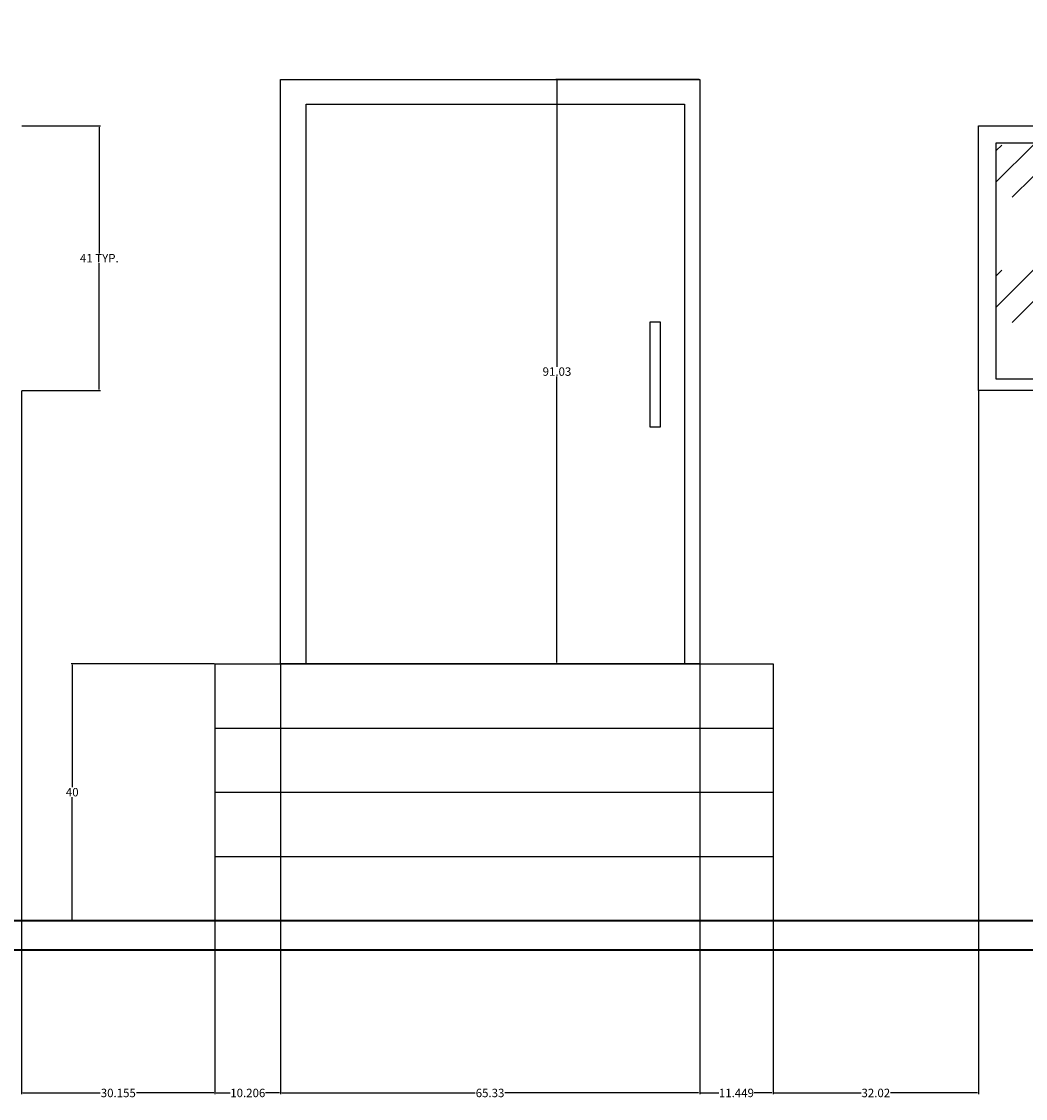
# Model space of a CAD drawing. Units: inches. Extents: x 30 to 515, y 94 to 489.
# Tile 4 of 7: x 202 to 358, y 94 to 262. Entities that reach past the tile are written whole.
import ezdxf

# ---------------------------------------------------------------- set-up
doc = ezdxf.new("R2010")
doc.units = ezdxf.units.IN
doc.header["$MEASUREMENT"] = 0
for name, color, linetype, lineweight in [('A-ANNO-DIMS', 2, 'Continuous', 18), ('A-DOOR', 4, 'Continuous', 25), ('A-FLOR-STRS', 3, 'Continuous', 25), ('A-GLAZ', 4, 'Continuous', 25), ('A-GLAZ-PATT', 8, 'Continuous', 13), ('A-WALL', 7, 'Continuous', 35)]:
    doc.layers.add(name, color=color, linetype=linetype, lineweight=lineweight)
doc.styles.get("Standard").update_dxf_attribs({"font": 'arial.ttf'})
doc.dimstyles.get("Standard").update_dxf_attribs({"dimtxt": 1.3125, "dimasz": 0.18, "dimexe": 0.18, "dimexo": 0.0625, "dimgap": 0.09, "dimtad": 0, "dimtih": 1, "dimtoh": 1, "dimdec": 4, "dimzin": 0, "dimdsep": 46, "dimlunit": 4, "dimtxsty": 'Standard', "dimcen": 0.09, "dimadec": 0, "dimazin": 0, "dimtfac": 1, "dimtdec": 4, "dimtofl": 0, "dimtmove": 0, "dimatfit": 3, "dimfxl": 1, "dimtolj": 1, "dimtzin": 0, "dimarcsym": 0})

# ---------------------------------------------------------------- blocks, each defined once
blk = doc.blocks.new('WIN-1100-DBL')
for points in [[(0, 41.22), (80.81, 41.22), (80.81, 0), (0, 0)], [(2.73, 38.58), (38.51, 38.58), (38.51, 1.75), (2.73, 1.75)], [(42.07, 38.58), (77.85, 38.58), (77.85, 1.75), (42.07, 1.75)], [(36.99, 20.89), (37.45, 20.89), (37.45, 13.69), (36.99, 13.69)], [(43.35, 20.89), (43.81, 20.89), (43.81, 13.69), (43.35, 13.69)]]:
    blk.add_lwpolyline(points, close=True)
blk = doc.blocks.new('*D3')
at = {"layer": 'A-ANNO-DIMS', "color": 0, "lineweight": -2, "transparency": 16777216}
for p, q in [((201.86, 245.32), (214.1, 245.32)), ((213.92, 245.14), (213.92, 225.45)), ((213.92, 204.27), (213.92, 223.96)), ((201.86, 204.09), (214.1, 204.09))]:
    blk.add_line(p, q, dxfattribs=at)
at = {"layer": 'A-ANNO-DIMS', "color": 0, "transparency": 16777216}
for points in [[(213.89, 245.14), (213.95, 245.14), (213.92, 245.32)], [(213.89, 204.27), (213.95, 204.27), (213.92, 204.09)]]:
    blk.add_solid(points, dxfattribs=at)
at = {"layer": 'Defpoints', "color": 0, "transparency": 16777216}
for p in [(201.8, 245.32), (213.92, 245.32), (201.8, 204.09)]:
    blk.add_point(p, dxfattribs=at)
at = {"layer": 'A-ANNO-DIMS', "color": 0, "transparency": 16777216, "insert": (213.92, 224.71), "char_height": 1.3125, "attachment_point": 5}
blk.add_mtext('\\A1;41 TYP.', dxfattribs=at)
blk = doc.blocks.new('*D8')
at = {"layer": 'A-ANNO-DIMS', "color": 0, "lineweight": -2, "transparency": 16777216}
for p, q in [((201.8, 204.03), (201.8, 94.5)), ((231.95, 121.47), (231.95, 94.5)), ((201.98, 94.68), (214.06, 94.68)), ((231.77, 94.68), (219.69, 94.68))]:
    blk.add_line(p, q, dxfattribs=at)
at = {"layer": 'A-ANNO-DIMS', "color": 0, "transparency": 16777216}
for points in [[(201.98, 94.71), (201.98, 94.65), (201.8, 94.68)], [(231.77, 94.71), (231.77, 94.65), (231.95, 94.68)]]:
    blk.add_solid(points, dxfattribs=at)
at = {"layer": 'Defpoints', "color": 0, "transparency": 16777216}
for p in [(201.8, 204.09), (231.95, 121.53), (231.95, 94.68)]:
    blk.add_point(p, dxfattribs=at)
at = {"layer": 'A-ANNO-DIMS', "color": 0, "transparency": 16777216, "insert": (216.88, 94.68), "char_height": 1.312, "attachment_point": 5}
blk.add_mtext('\\A1;30.155', dxfattribs=at)
blk = doc.blocks.new('*D9')
at = {"layer": 'A-ANNO-DIMS', "color": 0, "lineweight": -2, "transparency": 16777216}
for p, q in [((242.16, 161.47), (242.16, 94.5)), ((231.95, 121.47), (231.95, 94.5)), ((232.13, 94.68), (234.3, 94.68)), ((241.98, 94.68), (239.81, 94.68))]:
    blk.add_line(p, q, dxfattribs=at)
at = {"layer": 'A-ANNO-DIMS', "color": 0, "transparency": 16777216}
for points in [[(232.13, 94.71), (232.13, 94.65), (231.95, 94.68)], [(241.98, 94.71), (241.98, 94.65), (242.16, 94.68)]]:
    blk.add_solid(points, dxfattribs=at)
at = {"layer": 'Defpoints', "color": 0, "transparency": 16777216}
for p in [(242.16, 161.53), (231.95, 121.53), (242.16, 94.68)]:
    blk.add_point(p, dxfattribs=at)
at = {"layer": 'A-ANNO-DIMS', "color": 0, "transparency": 16777216, "insert": (237.06, 94.68), "char_height": 1.312, "attachment_point": 5}
blk.add_mtext('\\A1;10.206', dxfattribs=at)
blk = doc.blocks.new('*D10')
at = {"layer": 'A-ANNO-DIMS', "color": 0, "lineweight": -2, "transparency": 16777216}
for p, q in [((242.16, 161.47), (242.16, 94.5)), ((307.49, 161.47), (307.49, 94.5)), ((242.34, 94.68), (272.51, 94.68)), ((307.31, 94.68), (277.13, 94.68))]:
    blk.add_line(p, q, dxfattribs=at)
at = {"layer": 'A-ANNO-DIMS', "color": 0, "transparency": 16777216}
for points in [[(242.34, 94.71), (242.34, 94.65), (242.16, 94.68)], [(307.31, 94.71), (307.31, 94.65), (307.49, 94.68)]]:
    blk.add_solid(points, dxfattribs=at)
at = {"layer": 'Defpoints', "color": 0, "transparency": 16777216}
for p in [(242.16, 161.53), (307.49, 161.53), (307.49, 94.68)]:
    blk.add_point(p, dxfattribs=at)
at = {"layer": 'A-ANNO-DIMS', "color": 0, "transparency": 16777216, "insert": (274.82, 94.68), "char_height": 1.312, "attachment_point": 5}
blk.add_mtext('\\A1;65.33', dxfattribs=at)
blk = doc.blocks.new('*D11')
at = {"layer": 'A-ANNO-DIMS', "color": 0, "lineweight": -2, "transparency": 16777216}
for p, q in [((307.49, 161.47), (307.49, 94.5)), ((318.93, 121.47), (318.93, 94.5)), ((307.67, 94.68), (310.46, 94.68)), ((318.75, 94.68), (315.96, 94.68))]:
    blk.add_line(p, q, dxfattribs=at)
at = {"layer": 'A-ANNO-DIMS', "color": 0, "transparency": 16777216}
for points in [[(307.67, 94.71), (307.67, 94.65), (307.49, 94.68)], [(318.75, 94.71), (318.75, 94.65), (318.93, 94.68)]]:
    blk.add_solid(points, dxfattribs=at)
at = {"layer": 'Defpoints', "color": 0, "transparency": 16777216}
for p in [(307.49, 161.53), (318.93, 121.53), (318.93, 94.68)]:
    blk.add_point(p, dxfattribs=at)
at = {"layer": 'A-ANNO-DIMS', "color": 0, "transparency": 16777216, "insert": (313.21, 94.68), "char_height": 1.312, "attachment_point": 5}
blk.add_mtext('\\A1;11.449', dxfattribs=at)
blk = doc.blocks.new('*D12')
at = {"layer": 'A-ANNO-DIMS', "color": 0, "lineweight": -2, "transparency": 16777216}
for p, q in [((350.95, 204.03), (350.95, 94.5)), ((318.93, 121.47), (318.93, 94.5)), ((319.11, 94.68), (332.65, 94.68)), ((350.77, 94.68), (337.24, 94.68))]:
    blk.add_line(p, q, dxfattribs=at)
at = {"layer": 'A-ANNO-DIMS', "color": 0, "transparency": 16777216}
for points in [[(319.11, 94.71), (319.11, 94.65), (318.93, 94.68)], [(350.77, 94.71), (350.77, 94.65), (350.95, 94.68)]]:
    blk.add_solid(points, dxfattribs=at)
at = {"layer": 'Defpoints', "color": 0, "transparency": 16777216}
for p in [(350.95, 204.09), (318.93, 121.53), (350.95, 94.68)]:
    blk.add_point(p, dxfattribs=at)
at = {"layer": 'A-ANNO-DIMS', "color": 0, "transparency": 16777216, "insert": (334.94, 94.68), "char_height": 1.312, "attachment_point": 5}
blk.add_mtext('\\A1;32.02', dxfattribs=at)
blk = doc.blocks.new('*D28')
at = {"layer": 'A-ANNO-DIMS', "color": 0, "lineweight": -2, "transparency": 16777216}
for p, q in [((231.89, 161.53), (209.52, 161.53)), ((209.7, 161.35), (209.7, 142.29)), ((209.7, 121.71), (209.7, 140.77)), ((231.89, 121.53), (209.52, 121.53))]:
    blk.add_line(p, q, dxfattribs=at)
at = {"layer": 'A-ANNO-DIMS', "color": 0, "transparency": 16777216}
for points in [[(209.67, 161.35), (209.73, 161.35), (209.7, 161.53)], [(209.67, 121.71), (209.73, 121.71), (209.7, 121.53)]]:
    blk.add_solid(points, dxfattribs=at)
at = {"layer": 'Defpoints', "color": 0, "transparency": 16777216}
for p in [(209.7, 161.53), (231.95, 161.53), (231.95, 121.53)]:
    blk.add_point(p, dxfattribs=at)
at = {"layer": 'A-ANNO-DIMS', "color": 0, "transparency": 16777216, "insert": (209.7, 141.53), "char_height": 1.312, "attachment_point": 5}
blk.add_mtext('\\A1;40', dxfattribs=at)
blk = doc.blocks.new('*D29')
at = {"layer": 'A-ANNO-DIMS', "color": 0, "lineweight": -2, "transparency": 16777216}
for p, q in [((307.42, 252.56), (285.06, 252.56)), ((285.24, 252.38), (285.24, 207.81)), ((285.24, 161.71), (285.24, 206.28)), ((307.42, 161.53), (285.06, 161.53))]:
    blk.add_line(p, q, dxfattribs=at)
at = {"layer": 'A-ANNO-DIMS', "color": 0, "transparency": 16777216}
for points in [[(285.21, 252.38), (285.27, 252.38), (285.24, 252.56)], [(285.21, 161.71), (285.27, 161.71), (285.24, 161.53)]]:
    blk.add_solid(points, dxfattribs=at)
at = {"layer": 'Defpoints', "color": 0, "transparency": 16777216}
for p in [(285.24, 252.56), (307.49, 252.56), (307.49, 161.53)]:
    blk.add_point(p, dxfattribs=at)
at = {"layer": 'A-ANNO-DIMS', "color": 0, "transparency": 16777216, "insert": (285.24, 207.05), "char_height": 1.312, "attachment_point": 5}
blk.add_mtext('\\A1;91.03', dxfattribs=at)

msp = doc.modelspace()

# ---------------------------------------------------------------- hatches: boundary and pattern name
at = {"layer": 'A-GLAZ-PATT'}
h = msp.add_hatch(dxfattribs=at)
h.set_pattern_fill('GOST_GLASS', color=256, scale=2.3)
h.set_pattern_definition([(45, (0, 0), (19.51615, 0), [11.5, -16.1]), (45, (4.879, 0), (19.51615, 0), [4.6, -23]), (45, (0, 4.879), (19.51615, 0), [4.6, -23])])
h.paths.add_polyline_path([(141.7277, 354.4489), (122.2758, 354.4489), (122.2758, 330.4708), (141.7277, 330.4708)])
h.paths.add_polyline_path([(124.1475, 338.9533), (123.2785, 338.9533), (123.2785, 345.0981), (124.1475, 345.0981)], flags=16)
h.paths.add_polyline_path([(120.7384, 354.4489), (101.2865, 354.4489), (101.2865, 330.4708), (120.7384, 330.4708)])
h.paths.add_polyline_path([(119.0673, 338.9533), (119.0673, 345.0981), (119.9363, 345.0981), (119.9363, 338.9533)], flags=16)
h.paths.add_polyline_path([(159.5032, 242.6758), (123.7159, 242.6758), (123.7159, 205.8458), (159.5032, 205.8458)])
h.paths.add_polyline_path([(157.9822, 224.9831), (158.4447, 224.9831), (158.4447, 217.7871), (157.9822, 217.7871)], flags=16)
h.paths.add_polyline_path([(198.8424, 242.6758), (163.0551, 242.6758), (163.0551, 205.8458), (198.8424, 205.8458)])
h.paths.add_polyline_path([(164.8004, 224.9831), (164.8004, 217.7871), (164.3379, 217.7871), (164.3379, 224.9831)], flags=16)
h.paths.add_polyline_path([(389.467, 242.6758), (353.6798, 242.6758), (353.6798, 205.8458), (389.467, 205.8458)])
h.paths.add_polyline_path([(387.946, 224.9831), (388.4085, 224.9831), (388.4085, 217.7871), (387.946, 217.7871)], flags=16)
h.paths.add_polyline_path([(428.8062, 242.6758), (393.0189, 242.6758), (393.0189, 205.8458), (428.8062, 205.8458)])
h.paths.add_polyline_path([(394.7642, 224.9831), (394.7642, 217.7871), (394.3017, 217.7871), (394.3017, 224.9831)], flags=16)

# ---------------------------------------------------------------- linework, layer by layer
at = {"layer": 'A-DOOR'}
for points in [[(242.1589, 252.5624), (307.4854, 252.5624), (307.4854, 161.5281), (242.1589, 161.5281)], [(246.1679, 248.7129), (305.1403, 248.7129), (305.1403, 161.5281), (246.1679, 161.5281)], [(299.7732, 214.7924), (301.3196, 214.7924), (301.3196, 198.3757), (299.7732, 198.3757)]]:
    msp.add_lwpolyline(points, close=True, dxfattribs=at)
at = {"layer": 'A-FLOR-STRS'}
for p, q in [((231.9527, 151.5281), (231.9527, 161.5281)), ((231.9527, 161.5281), (318.9339, 161.5281)), ((318.9339, 161.5281), (318.9339, 151.5281)), ((231.9527, 141.5281), (231.9527, 151.5281)), ((231.9527, 151.5281), (318.9339, 151.5281)), ((318.9339, 151.5281), (318.9339, 141.5281)), ((231.9527, 131.5281), (231.9527, 141.5281)), ((231.9527, 141.5281), (318.9339, 141.5281)), ((318.9339, 141.5281), (318.9339, 131.5281)), ((231.9527, 121.5281), (231.9527, 131.5281)), ((231.9527, 131.5281), (318.9339, 131.5281)), ((318.9339, 131.5281), (318.9339, 121.5281))]:
    msp.add_line(p, q, dxfattribs=at)
at = {"layer": 'A-WALL'}
for p, q in [((67.017, 121.5281), (448.0511, 121.5281)), ((448.0511, 116.9344), (67.017, 116.9344))]:
    msp.add_line(p, q, dxfattribs=at)

# ---------------------------------------------------------------- block references
at = {"layer": 'A-GLAZ'}
msp.add_blockref('WIN-1100-DBL', (350.9538, 204.094), dxfattribs=at)

# ---------------------------------------------------------------- dimensions: what is measured, and where the dimension line sits
at = {"layer": 'A-ANNO-DIMS'}
for base, p1, p2, override, picture, middle in [((285.2354, 252.5624), (307.4854, 161.5281), (307.4854, 252.5624), {"dimdec": 2, "dimlfac": 1, "dimrnd": 0, "dimzin": 0, "dimdsep": 46, "dimlunit": 2}, '*D29', (285.2354, 207.0452)), ((209.7027, 161.5281), (231.9527, 121.5281), (231.9527, 161.5281), {"dimdec": 0, "dimlfac": 1, "dimrnd": 0, "dimzin": 0, "dimdsep": 46, "dimlunit": 2}, '*D28', (209.7027, 141.5281))]:
    dim = msp.add_linear_dim(base=base, p1=p1, p2=p2, angle=90, dimstyle='Standard', override=override, dxfattribs=at)
    dim.commit()
    dim.dimension.update_dxf_attribs({"geometry": picture, "text_midpoint": middle})
dim = msp.add_linear_dim(base=(213.9186, 245.317), p1=(201.7974, 204.0939), p2=(201.7974, 245.317), angle=90, text='<> TYP.', dimstyle='Standard', override={"dimdec": 0, "dimlfac": 1, "dimrnd": 0, "dimzin": 0, "dimdsep": 46, "dimlunit": 2}, dxfattribs=at)
dim.commit()
dim.dimension.update_dxf_attribs({"geometry": '*D3', "text_midpoint": (213.9186, 224.7054)})
for base, p1, p2, override, picture, middle in [((231.9527, 94.6844), (201.7974, 204.0939), (231.9527, 121.5281), {"dimdec": 3, "dimlfac": 1, "dimrnd": 0, "dimzin": 0, "dimdsep": 46, "dimlunit": 2}, '*D8', (216.8751, 94.6844)), ((350.9536, 94.6844), (318.9339, 121.5281), (350.9536, 204.0939), {"dimdec": 2, "dimlfac": 1, "dimrnd": 0, "dimzin": 0, "dimdsep": 46, "dimlunit": 2}, '*D12', (334.9438, 94.6844)), ((242.1589, 94.6844), (231.9527, 121.5281), (242.1589, 161.5281), {"dimdec": 3, "dimlfac": 1, "dimrnd": 0, "dimzin": 0, "dimdsep": 46, "dimlunit": 2}, '*D9', (237.0558, 94.6844)), ((307.4854, 94.6844), (242.1589, 161.5281), (307.4854, 161.5281), {"dimdec": 2, "dimlfac": 1, "dimrnd": 0, "dimzin": 0, "dimdsep": 46, "dimlunit": 2}, '*D10', (274.8222, 94.6844)), ((318.93395, 94.68438), (307.48544, 161.52806), (318.93395, 121.52806), {"dimdec": 3, "dimlfac": 1, "dimrnd": 0, "dimzin": 0, "dimdsep": 46, "dimlunit": 2}, '*D11', (313.20969, 94.68438))]:
    dim = msp.add_linear_dim(base=base, p1=p1, p2=p2, dimstyle='Standard', override=override, dxfattribs=at)
    dim.commit()
    dim.dimension.update_dxf_attribs({"geometry": picture, "text_midpoint": middle})

doc.saveas('drawing.dxf')
